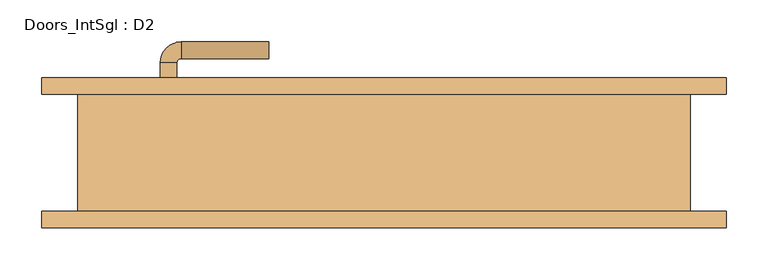
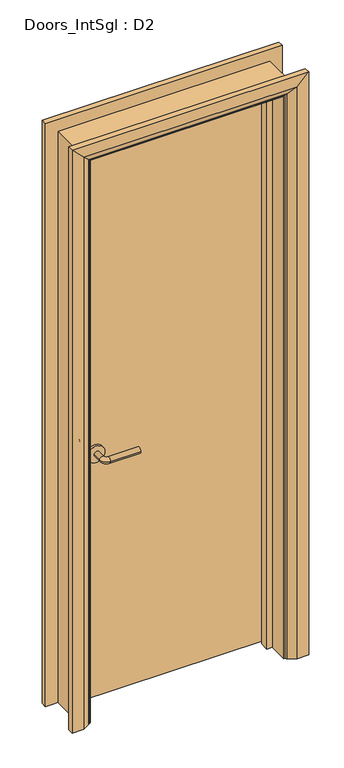
"""IFC4 building model written with IfcOpenShell, lengths in millimetres: door geometry, Doors_IntSgl : D2."""

from ifc_helpers import new_model, si_unit, point, frame, frame_2d, origin, place, context, project, spatial, polyline, circle_curve, ellipse_curve, trimmed, segment, composite_curve, outline, extrude, faceted_brep, source, transform, mapped, element, save
from ifc_brep_helpers import plane_surface, cylinder_surface, revolved_surface, advanced_brep


def doors_intsgl_d2_e5ed4415(model_context):
    return source(origin(), model_context, "Body", "SolidModel", [
        advanced_brep(
        [(-268.0, 24.0, 900.0), (-248.0, 24.0, 900.0), (-248.0, -6.0, 900.0), (-268.0, -6.0, 900.0), (-243.0, -11.0, 900.0), (-243.0, -31.0, 900.0), (-138.0, -31.0, 900.0), (-138.0, -11.0, 900.0)],
        [
            (0, 1, circle_curve(frame((-258.0, 24.0, 900.0), z_axis=(0.0, 1.0, 0.0), x_axis=(1.0, 0.0, 0.0)), 10.0)),
            (1, 0, circle_curve(frame((-258.0, 24.0, 900.0), z_axis=(0.0, 1.0, 0.0), x_axis=(1.0, 0.0, 0.0)), 10.0)),
            (1, 2),
            (2, 3, circle_curve(frame((-258.0, -6.0, 900.0), z_axis=(0.0, 1.0, 0.0), x_axis=(1.0, 0.0, 0.0)), 10.0)),
            (3, 0),
            (3, 2, circle_curve(frame((-258.0, -6.0, 900.0), z_axis=(0.0, 1.0, 0.0), x_axis=(1.0, 0.0, 0.0)), 10.0)),
            (4, 5, circle_curve(frame((-243.0, -21.0, 900.0), z_axis=(-1.0, 0.0, 0.0), x_axis=(0.0, 1.0, 0.0)), 10.0)),
            (5, 3, circle_curve(frame((-243.0, -6.0, 900.0), z_axis=(0.0, 0.0, -1.0), x_axis=(-1.0, 0.0, 0.0)), 25.0)),
            (2, 4, circle_curve(frame((-243.0, -6.0, 900.0), z_axis=(0.0, 0.0, 1.0), x_axis=(-1.0, 0.0, 0.0)), 5.0)),
            (5, 4, circle_curve(frame((-243.0, -21.0, 900.0), z_axis=(-1.0, 0.0, 0.0), x_axis=(0.0, 1.0, 0.0)), 10.0)),
            (6, 7, circle_curve(frame((-138.0, -21.0, 900.0), z_axis=(1.0, 0.0, 0.0), x_axis=(0.0, 1.0, 0.0)), 10.0)),
            (7, 6, circle_curve(frame((-138.0, -21.0, 900.0), z_axis=(1.0, 0.0, 0.0), x_axis=(0.0, 1.0, 0.0)), 10.0)),
            (4, 7),
            (6, 5),
        ],
        [
            plane_surface(frame((-258.0, 24.0, 900.0), z_axis=(0.0, 1.0, 0.0), x_axis=(0.0, 0.0, 1.0))),
            cylinder_surface(frame((-258.0, 24.0, 900.0), z_axis=(0.0, 1.0, 0.0), x_axis=(1.0, 0.0, 0.0)), 10.0),
            revolved_surface(trimmed(ellipse_curve(frame((-258.0, -6.0, 900.0), z_axis=(0.0, -1.0, 0.0), x_axis=(1.0, 0.0, 0.0)), 10.0, 10.0), [point((-268.0, -6.0, 900.0))], [point((-248.0, -6.0, 900.0))], True, "CARTESIAN"), (-243.0, -6.0, 900.0), (0.0, 0.0, -1.0)),
            revolved_surface(trimmed(ellipse_curve(frame((-258.0, -6.0, 900.0), z_axis=(0.0, -1.0, 0.0), x_axis=(1.0, 0.0, 0.0)), 10.0, 10.0), [point((-248.0, -6.0, 900.0))], [point((-268.0, -6.0, 900.0))], True, "CARTESIAN"), (-243.0, -6.0, 900.0), (0.0, 0.0, -1.0)),
            plane_surface(frame((-138.0, -21.0, 900.0), z_axis=(1.0, 0.0, 0.0), x_axis=(0.0, 0.0, 1.0))),
            cylinder_surface(frame((-243.0, -21.0, 900.0), z_axis=(-1.0, 0.0, 0.0), x_axis=(0.0, 1.0, 0.0)), 10.0),
        ],
        [
            (0, [[1, 2]]),
            (1, [[3, 4, 5, -2]]),
            (1, [[-5, 6, -3, -1]]),
            (2, [[7, 8, -4, 9]]),
            (3, [[10, -9, -6, -8]]),
            (4, [[11, 12]]),
            (5, [[13, -11, 14, -7]]),
            (5, [[-14, -12, -13, -10]]),
        ],
    ),
        extrude(outline(composite_curve([segment(trimmed(circle_curve(frame_2d((900.0, -260.5)), 30.0), [point((900.0, -290.5))], [point((900.0, -230.5))], False, "CARTESIAN"), True, "CONTINUOUS"), segment(trimmed(circle_curve(frame_2d((900.0, -260.5)), 30.0), [point((900.0, -230.5))], [point((900.0, -290.5))], False, "CARTESIAN"), True, "CONTINUOUS")], self_intersect=False)), frame((0.0, 24.0, 0.0), z_axis=(0.0, 1.0, 0.0), x_axis=(0.0, 0.0, 1.0)), (0.0, 0.0, 1.0), 8.0),
        advanced_brep(
        [(-268.0, 78.0, 900.0), (-248.0, 78.0, 900.0), (-268.0, 108.0, 900.0), (-248.0, 108.0, 900.0), (-243.0, 113.0, 900.0), (-243.0, 133.0, 900.0), (-138.0, 133.0, 900.0), (-138.0, 113.0, 900.0)],
        [
            (0, 1, circle_curve(frame((-258.0, 78.0, 900.0), z_axis=(0.0, -1.0, 0.0), x_axis=(1.0, 0.0, 0.0)), 10.0)),
            (1, 0, circle_curve(frame((-258.0, 78.0, 900.0), z_axis=(0.0, -1.0, 0.0), x_axis=(1.0, 0.0, 0.0)), 10.0)),
            (0, 2),
            (2, 3, circle_curve(frame((-258.0, 108.0, 900.0), z_axis=(0.0, -1.0, 0.0), x_axis=(1.0, 0.0, 0.0)), 10.0)),
            (3, 1),
            (3, 2, circle_curve(frame((-258.0, 108.0, 900.0), z_axis=(0.0, -1.0, 0.0), x_axis=(1.0, 0.0, 0.0)), 10.0)),
            (4, 3, circle_curve(frame((-243.0, 108.0, 900.0), z_axis=(0.0, 0.0, 1.0), x_axis=(-1.0, 0.0, 0.0)), 5.0)),
            (2, 5, circle_curve(frame((-243.0, 108.0, 900.0), z_axis=(0.0, 0.0, -1.0), x_axis=(-1.0, 0.0, 0.0)), 25.0)),
            (5, 4, circle_curve(frame((-243.0, 123.0, 900.0), z_axis=(-1.0, 0.0, 0.0), x_axis=(0.0, -1.0, 0.0)), 10.0)),
            (4, 5, circle_curve(frame((-243.0, 123.0, 900.0), z_axis=(-1.0, 0.0, 0.0), x_axis=(0.0, -1.0, 0.0)), 10.0)),
            (6, 7, circle_curve(frame((-138.0, 123.0, 900.0), z_axis=(1.0, 0.0, 0.0), x_axis=(0.0, -1.0, 0.0)), 10.0)),
            (7, 6, circle_curve(frame((-138.0, 123.0, 900.0), z_axis=(1.0, 0.0, 0.0), x_axis=(0.0, -1.0, 0.0)), 10.0)),
            (5, 6),
            (7, 4),
        ],
        [
            plane_surface(frame((-258.0, 78.0, 900.0), z_axis=(0.0, -1.0, 0.0), x_axis=(0.0, 0.0, 1.0))),
            cylinder_surface(frame((-258.0, 78.0, 900.0), z_axis=(0.0, -1.0, 0.0), x_axis=(1.0, 0.0, 0.0)), 10.0),
            revolved_surface(trimmed(ellipse_curve(frame((-258.0, 108.0, 900.0), z_axis=(0.0, -1.0, 0.0), x_axis=(1.0, 0.0, 0.0)), 10.0, 10.0), [point((-268.0, 108.0, 900.0))], [point((-248.0, 108.0, 900.0))], True, "CARTESIAN"), (-243.0, 108.0, 900.0), (0.0, 0.0, -1.0)),
            revolved_surface(trimmed(ellipse_curve(frame((-258.0, 108.0, 900.0), z_axis=(0.0, -1.0, 0.0), x_axis=(1.0, 0.0, 0.0)), 10.0, 10.0), [point((-248.0, 108.0, 900.0))], [point((-268.0, 108.0, 900.0))], True, "CARTESIAN"), (-243.0, 108.0, 900.0), (0.0, 0.0, -1.0)),
            plane_surface(frame((-138.0, 123.0, 900.0), z_axis=(1.0, 0.0, 0.0), x_axis=(0.0, 0.0, 1.0))),
            cylinder_surface(frame((-243.0, 123.0, 900.0), z_axis=(-1.0, 0.0, 0.0), x_axis=(0.0, -1.0, 0.0)), 10.0),
        ],
        [
            (0, [[1, 2]]),
            (1, [[-1, 3, 4, 5]]),
            (1, [[-2, -5, 6, -3]]),
            (2, [[7, -4, 8, 9]]),
            (3, [[-8, -6, -7, 10]]),
            (4, [[11, 12]]),
            (5, [[-9, 13, -12, 14]]),
            (5, [[-10, -14, -11, -13]]),
        ],
    ),
        extrude(outline(composite_curve([segment(trimmed(circle_curve(frame_2d((900.0, -260.5)), 30.0), [point((900.0, -290.5))], [point((900.0, -230.5))], False, "CARTESIAN"), True, "CONTINUOUS"), segment(trimmed(circle_curve(frame_2d((900.0, -260.5)), 30.0), [point((900.0, -230.5))], [point((900.0, -290.5))], False, "CARTESIAN"), True, "CONTINUOUS")], self_intersect=False)), frame((0.0, 70.0, 0.0), z_axis=(0.0, 1.0, 0.0), x_axis=(0.0, 0.0, 1.0)), (0.0, 0.0, 1.0), 8.0),
        extrude(outline(polyline([(333.0, 32.0), (-333.0, 32.0), (-333.0, 70.0), (333.0, 70.0), (333.0, 32.0)])), frame((0.0, 0.0, 8.0), z_axis=(0.0, 0.0, 1.0), x_axis=(1.0, 0.0, 0.0)), (0.0, 0.0, 1.0), 2050.0),
        advanced_brep(
        [(410.0, 90.0, 0.0), (410.0, 70.0, 0.0), (340.0, 70.0, 0.0), (344.0, 76.0, 0.0), (370.0, 90.0, 0.0), (410.0, 90.0, 2135.0), (410.0, 70.0, 2135.0), (-410.0, 70.0, 2135.0), (-410.0, 70.0, 0.0), (-340.0, 70.0, 0.0), (-340.0, 70.0, 2065.0), (340.0, 70.0, 2065.0), (344.0, 76.0, 2069.0), (370.0, 90.0, 2095.0), (-370.0, 90.0, 2095.0), (-370.0, 90.0, 0.0), (-410.0, 90.0, 0.0), (-410.0, 90.0, 2135.0), (-344.0, 76.0, 0.0), (-344.0, 76.0, 2069.0)],
        [
            (0, 1),
            (1, 2),
            (2, 3, circle_curve(frame((348.0, 69.0, 0.0), z_axis=(0.0, 0.0, -1.0), x_axis=(1.0, 0.0, 0.0)), 8.0622577)),
            (3, 4),
            (4, 0),
            (0, 5),
            (5, 6),
            (6, 1),
            (6, 7),
            (7, 8),
            (8, 9),
            (9, 10),
            (10, 11),
            (11, 2),
            (11, 12, ellipse_curve(frame((348.0, 69.0, 2073.0), z_axis=(0.7071067811865475, 0.0, -0.7071067811865475), x_axis=(-0.7071067811865474, 0.0, -0.7071067811865476)), 11.4017543, 8.0622577)),
            (12, 3),
            (12, 13),
            (13, 4),
            (13, 14),
            (14, 15),
            (15, 16),
            (16, 17),
            (17, 5),
            (7, 17),
            (16, 8),
            (15, 18),
            (18, 9, circle_curve(frame((-348.0, 69.0, 0.0), z_axis=(0.0, 0.0, -1.0), x_axis=(-1.0, 0.0, 0.0)), 8.0622577)),
            (19, 10, ellipse_curve(frame((-348.0, 69.0, 2073.0), z_axis=(-0.7071067811865475, 0.0, -0.7071067811865475), x_axis=(-0.7071067811865474, 0.0, 0.7071067811865476)), 11.4017543, 8.0622577)),
            (18, 19),
            (14, 19),
            (19, 12),
        ],
        [
            plane_surface(frame((340.0, 70.0, 0.0), z_axis=(0.0, 0.0, -1.0), x_axis=(0.0, -1.0, 0.0))),
            plane_surface(frame((410.0, 90.0, 0.0), z_axis=(1.0, 0.0, 0.0), x_axis=(0.0, 0.0, 1.0))),
            plane_surface(frame((410.0, 70.0, 0.0), z_axis=(0.0, -1.0, 0.0), x_axis=(0.0, 0.0, 1.0))),
            cylinder_surface(frame((348.0, 69.0, 0.0), z_axis=(0.0, 0.0, -1.0), x_axis=(1.0, 0.0, 0.0)), 8.0622577),
            plane_surface(frame((344.0, 76.0, 0.0), z_axis=(-0.4740998230350126, 0.880471099922178, 0.0), x_axis=(0.0, 0.0, 1.0))),
            plane_surface(frame((370.0, 90.0, 0.0), z_axis=(0.0, 1.0, 0.0), x_axis=(0.0, 0.0, 1.0))),
            plane_surface(frame((-410.0, 90.0, 2135.0), z_axis=(-1.0, 0.0, 0.0), x_axis=(0.0, 0.0, -1.0))),
            plane_surface(frame((-340.0, 70.0, 0.0), z_axis=(0.0, 0.0, -1.0), x_axis=(0.0, -1.0, 0.0))),
            cylinder_surface(frame((-348.0, 69.0, 2065.0), z_axis=(0.0, 0.0, 1.0), x_axis=(-1.0, 0.0, 0.0)), 8.0622577),
            plane_surface(frame((-344.0, 76.0, 2069.0), z_axis=(0.47409982303501824, 0.8804710999221749, 0.0), x_axis=(0.0, 0.0, -1.0))),
            plane_surface(frame((410.0, 90.0, 2135.0), z_axis=(0.0, 0.0, 1.0), x_axis=(-1.0, 0.0, 0.0))),
            cylinder_surface(frame((340.0, 69.0, 2073.0), z_axis=(1.0, 0.0, 0.0), x_axis=(0.0, 0.0, 1.0)), 8.0622577),
            plane_surface(frame((344.0, 76.0, 2069.0), z_axis=(0.0, 0.8804710999221764, -0.4740998230350154), x_axis=(-1.0, 0.0, 0.0))),
        ],
        [
            (0, [[1, 2, 3, 4, 5]]),
            (1, [[-1, 6, 7, 8]]),
            (2, [[-2, -8, 9, 10, 11, 12, 13, 14]]),
            (3, [[-3, -14, 15, 16]]),
            (4, [[-4, -16, 17, 18]]),
            (5, [[-5, -18, 19, 20, 21, 22, 23, -6]]),
            (6, [[24, -22, 25, -10]]),
            (7, [[-21, 26, 27, -11, -25]]),
            (8, [[28, -12, -27, 29]]),
            (9, [[30, -29, -26, -20]]),
            (10, [[-7, -23, -24, -9]]),
            (11, [[-15, -13, -28, 31]]),
            (12, [[-17, -31, -30, -19]]),
        ],
    ),
        extrude(outline(polyline([(0.0, -335.0), (0.0, -316.0), (2041.0, -316.0), (2041.0, 316.0), (0.0, 316.0), (0.0, 335.0), (2060.0, 335.0), (2060.0, -335.0), (0.0, -335.0)])), frame((0.0, -2.0, 0.0), z_axis=(0.0, 1.0, 0.0), x_axis=(0.0, 0.0, 1.0)), (0.0, 0.0, 1.0), 32.0),
        advanced_brep(
        [(-410.0, -90.0, 0.0), (-410.0, -70.0, 0.0), (-340.0, -70.0, 0.0), (-344.0, -76.0, 0.0), (-370.0, -90.0, 0.0), (-410.0, -90.0, 2135.0), (-410.0, -70.0, 2135.0), (-340.0, -70.0, 2065.0), (-344.0, -76.0, 2069.0), (-370.0, -90.0, 2095.0), (410.0, -90.0, 0.0), (370.0, -90.0, 0.0), (344.0, -76.0, 0.0), (340.0, -70.0, 0.0), (410.0, -70.0, 0.0), (410.0, -90.0, 2135.0), (370.0, -90.0, 2095.0), (344.0, -76.0, 2069.0), (340.0, -70.0, 2065.0), (410.0, -70.0, 2135.0)],
        [
            (0, 1),
            (1, 2),
            (2, 3, circle_curve(frame((-348.0, -69.0, 0.0), z_axis=(0.0, 0.0, -1.0), x_axis=(-1.0, 0.0, 0.0)), 8.0622577)),
            (3, 4),
            (4, 0),
            (0, 5),
            (5, 6),
            (6, 1),
            (6, 7),
            (7, 2),
            (7, 8, ellipse_curve(frame((-348.0, -69.0, 2073.0), z_axis=(-0.7071067811865475, 0.0, -0.7071067811865475), x_axis=(0.7071067811865474, 0.0, -0.7071067811865476)), 11.4017543, 8.0622577)),
            (8, 3),
            (8, 9),
            (9, 4),
            (9, 5),
            (10, 11),
            (11, 12),
            (12, 13, circle_curve(frame((348.0, -69.0, 0.0), z_axis=(0.0, 0.0, -1.0), x_axis=(1.0, 0.0, 0.0)), 8.0622577)),
            (13, 14),
            (14, 10),
            (15, 16),
            (16, 11),
            (10, 15),
            (16, 17),
            (17, 12),
            (17, 18, ellipse_curve(frame((348.0, -69.0, 2073.0), z_axis=(0.7071067811865475, 0.0, -0.7071067811865475), x_axis=(0.7071067811865474, 0.0, 0.7071067811865476)), 11.4017543, 8.0622577)),
            (18, 13),
            (18, 19),
            (19, 14),
            (19, 15),
            (5, 15),
            (19, 6),
            (18, 7),
            (17, 8),
            (16, 9),
        ],
        [
            plane_surface(frame((-340.0, -142.8010989, 0.0), z_axis=(0.0, 0.0, -1.0), x_axis=(1.0, 0.0, 0.0))),
            plane_surface(frame((-410.0, -90.0, 0.0), z_axis=(-1.0, 0.0, 0.0), x_axis=(0.0, 0.0, 1.0))),
            plane_surface(frame((-410.0, -70.0, 0.0), z_axis=(0.0, 1.0, 0.0), x_axis=(0.0, 0.0, 1.0))),
            cylinder_surface(frame((-348.0, -69.0, 0.0), z_axis=(0.0, 0.0, -1.0), x_axis=(-1.0, 0.0, 0.0)), 8.0622577),
            plane_surface(frame((-344.0, -76.0, 0.0), z_axis=(0.4740998230350183, -0.8804710999221749, 0.0), x_axis=(0.0, 0.0, 1.0))),
            plane_surface(frame((-370.0, -90.0, 0.0), z_axis=(0.0, -1.0, 0.0), x_axis=(0.0, 0.0, 1.0))),
            plane_surface(frame((340.0, -142.8010989, 0.0), z_axis=(0.0, 0.0, -1.0), x_axis=(-1.0, 0.0, 0.0))),
            plane_surface(frame((370.0, -90.0, 2095.0), z_axis=(0.0, -1.0, 0.0), x_axis=(0.0, 0.0, -1.0))),
            plane_surface(frame((344.0, -76.0, 2069.0), z_axis=(-0.4740998230350183, -0.8804710999221749, 0.0), x_axis=(0.0, 0.0, -1.0))),
            cylinder_surface(frame((348.0, -69.0, 2065.0), z_axis=(0.0, 0.0, 1.0), x_axis=(1.0, 0.0, 0.0)), 8.0622577),
            plane_surface(frame((410.0, -70.0, 2135.0), z_axis=(0.0, 1.0, 0.0), x_axis=(0.0, 0.0, -1.0))),
            plane_surface(frame((410.0, -90.0, 2135.0), z_axis=(1.0, 0.0, 0.0), x_axis=(0.0, 0.0, -1.0))),
            plane_surface(frame((-410.0, -90.0, 2135.0), z_axis=(0.0, 0.0, 1.0), x_axis=(1.0, 0.0, 0.0))),
            plane_surface(frame((-410.0, -70.0, 2135.0), z_axis=(0.0, 1.0, 0.0), x_axis=(1.0, 0.0, 0.0))),
            cylinder_surface(frame((-340.0, -69.0, 2073.0), z_axis=(-1.0, 0.0, 0.0), x_axis=(0.0, 0.0, 1.0)), 8.0622577),
            plane_surface(frame((-344.0, -76.0, 2069.0), z_axis=(0.0, -0.8804710999221749, -0.4740998230350183), x_axis=(1.0, 0.0, 0.0))),
            plane_surface(frame((-370.0, -90.0, 2095.0), z_axis=(0.0, -1.0, 0.0), x_axis=(1.0, 0.0, 0.0))),
        ],
        [
            (0, [[1, 2, 3, 4, 5]]),
            (1, [[-1, 6, 7, 8]]),
            (2, [[-2, -8, 9, 10]]),
            (3, [[-3, -10, 11, 12]]),
            (4, [[-4, -12, 13, 14]]),
            (5, [[-5, -14, 15, -6]]),
            (6, [[16, 17, 18, 19, 20]]),
            (7, [[21, 22, -16, 23]]),
            (8, [[24, 25, -17, -22]]),
            (9, [[26, 27, -18, -25]]),
            (10, [[28, 29, -19, -27]]),
            (11, [[30, -23, -20, -29]]),
            (12, [[-7, 31, -30, 32]]),
            (13, [[-9, -32, -28, 33]]),
            (14, [[-11, -33, -26, 34]]),
            (15, [[-13, -34, -24, 35]]),
            (16, [[-15, -35, -21, -31]]),
        ],
    ),
        faceted_brep([(-335.0, 70.0, 0.0), (-335.0, -70.0, 0.0), (-367.0, -70.0, 0.0), (-367.0, 70.0, 0.0), (-335.0, 70.0, 2060.0), (-335.0, -70.0, 2060.0), (-367.0, -70.0, 2092.0), (-367.0, 70.0, 2092.0), (335.0, 70.0, 0.0), (367.0, 70.0, 0.0), (367.0, -70.0, 0.0), (335.0, -70.0, 0.0), (335.0, 70.0, 2060.0), (367.0, 70.0, 2092.0), (367.0, -70.0, 2092.0), (335.0, -70.0, 2060.0)], [[[0, 1, 2, 3]], [[1, 0, 4, 5]], [[2, 1, 5, 6]], [[3, 2, 6, 7]], [[0, 3, 7, 4]], [[8, 9, 10, 11]], [[12, 13, 9, 8]], [[13, 14, 10, 9]], [[14, 15, 11, 10]], [[15, 12, 8, 11]], [[5, 4, 12, 15]], [[6, 5, 15, 14]], [[7, 6, 14, 13]], [[4, 7, 13, 12]]]),
    ])


if __name__ == "__main__":
    model = new_model("IFC4")
    model_context = context("Model", 3, world=origin())
    ifc_project = project(units=[si_unit("LENGTHUNIT", "METRE", prefix="MILLI")], contexts=[model_context])
    site = spatial("IfcSite", under=ifc_project)
    building = spatial("IfcBuilding", under=site)
    placement = place(None, origin())
    doors_intsgl_d2_shape = doors_intsgl_d2_e5ed4415(model_context)
    element("IfcDoor", 1, ObjectType="Doors_IntSgl : D2", at=placement, inside=building, context=model_context, shape_type="MappedRepresentation", body=[
        mapped(doors_intsgl_d2_shape, transform((0.0, 0.0, 0.0), x_axis=(1.0, 0.0, 0.0), y_axis=(0.0, 1.0, 0.0), z_axis=(0.0, 0.0, 1.0))),
    ])
    save(model, "model.ifc")

# Revit data of these elements
# Type "Doors_IntSgl : D2"
#   Type Mark = "47"
#   Type Comments = "Internal Single"
#   Operation = "SingleSwingRight"
#   Manufacturer = "Revit"
#   Keynote = "L20"
#   Description = "Internal Single Door"
#   Analytic Construction = "Metal"
#   UnderCut = 8 mm
#   Tolerance = 2 mm
#   Thickness = 38 mm
#   Thermal Resistance (R) = 0.270117 (m²·K)/W
#   Structural Tolerance = 8 mm
#   StopDepth = 32 mm
#   Stop Thickness = 19 mm
#   Rough Width = 750 mm
#   Rough Height = 2100 mm
#   Height to Top Lock Rail = 1000 mm
#   Heat Transfer Coefficient (U) = 3.7021 W/(m²·K)
#   Handle Z Distance = 900 mm
#   Handle X Distance = 75 mm
#   Frame Thickness = 32 mm
#   Door Panel Width = 666 mm
#   Door Panel Thickness = 38 mm
#   Door Panel Offset = 0 mm
#   Height = 2100 mm
#   Width = 750 mm
#   Door Panel Height = 2050 mm
#   Architrave Setback = 5 mm
#   Vis - Ironmongery = yes
#   Material Ironmongery = Door - Handle
#   Material Frame = Door - Frame/Mullion (1)
#   Material Door = Door - Panel
#   Material Architrave = Door - Architrave
#   Visual Light Transmittance = 0
#   Solar Heat Gain Coefficient = 0
#   Function = (empty or 0)
#   Wall Closure = (empty or 0)
# Element 1 (IfcDoor, "Doors_IntSgl : D2")
#   Materials on its faces: "Door - Architrave", "Door - Handle", "Door - Frame/Mullion (1)", "Door - Panel"
# Materials
#   "Door - Handle": colour RGB 0 0 0, transparency 0, Keynote = "P21", Cost = 0
#   "Door - Frame/Mullion (1)": class "Wood", colour RGB 212 179 113, transparency 0, Keynote = "L20", Cost = 0
#   "Door - Panel": class "Wood", colour RGB 210 159 95, transparency 0, Keynote = "L20", Cost = 0
#   "Door - Architrave": class "Wood", colour RGB 154 90 5, transparency 0, Keynote = "P20", Cost = 0
